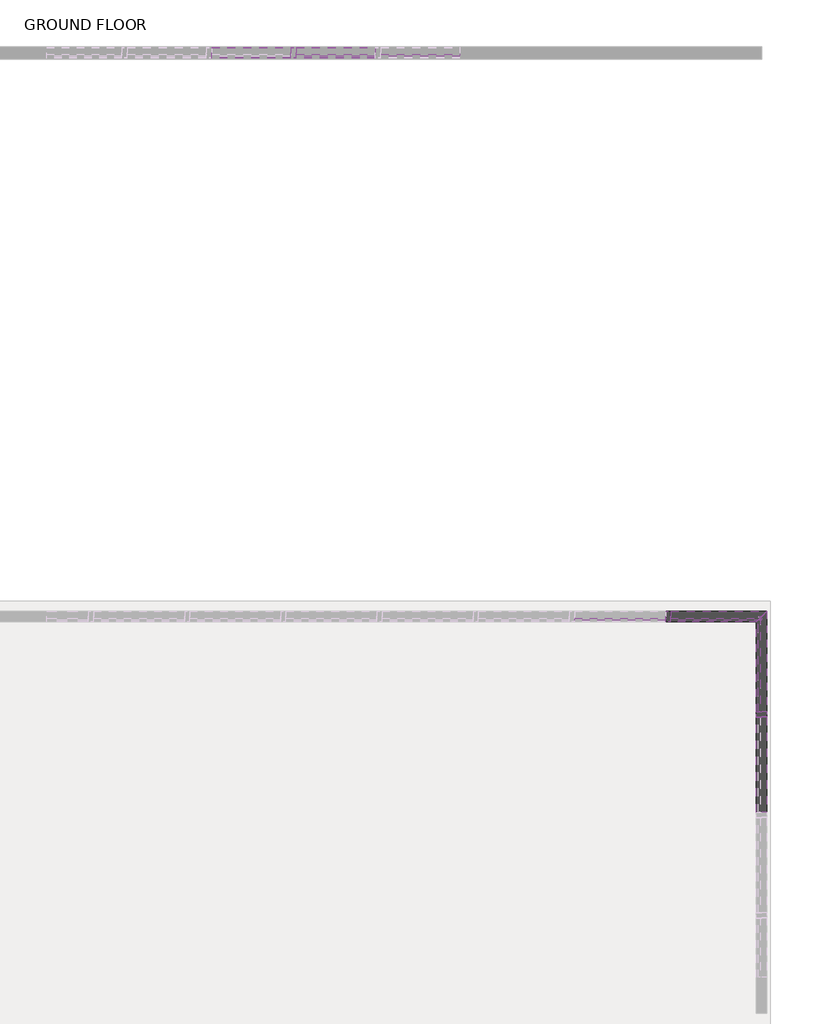
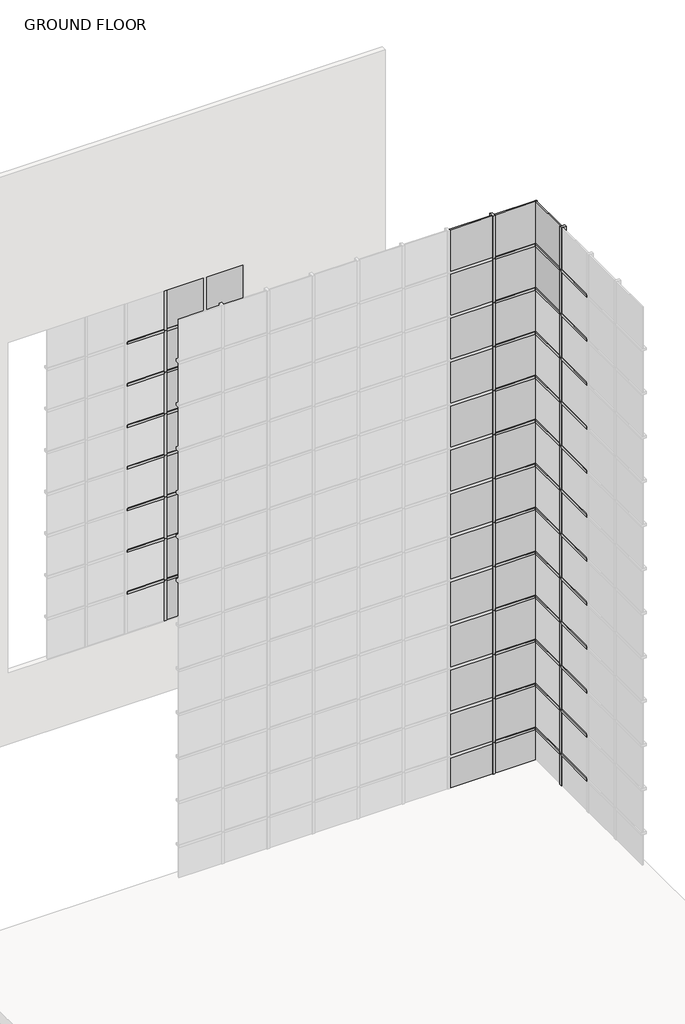
# One storey, part 14 of 16: 84 members, 44 plates.
"""IFC4 building model written with IfcOpenShell, lengths in millimetres."""

from ifc_helpers import new_model, si_unit, origin, place, context, project, spatial, transform, mapped, element, save
from components import member_b860638c, member_31fee25f, member_49b1bc66, member_1d29426d, member_637f24d3, member_76449a13, member_3df3cfcf, member_368818a6, system_panel_glazed_5cba32e5, system_panel_glazed_49652e9e, system_panel_glazed_6a711426

model = new_model("IFC4")

# Units and contexts
model_context = context("Model", 3, world=origin())
ifc_project = project(units=[si_unit("LENGTHUNIT", "METRE", prefix="MILLI")], contexts=[model_context])

# Site, building, storey
site = spatial("IfcSite", under=ifc_project)
building = spatial("IfcBuilding", under=site)
storey = spatial("IfcBuildingStorey", under=building, Name="GROUND FLOOR", Elevation=0.0)

# Members
placement = place(None, origin())
member_shape = member_b860638c(model_context)
element("IfcMember", 1, ObjectType="Rectangular Mullion : 2.5\" x 5\" rectangular", at=placement, inside=storey, context=model_context, shape_type="MappedRepresentation", body=[
    mapped(member_shape, transform((5962.6982466, 5184.6811965, 0.0), x_axis=(0.0, 1.0, 0.0), y_axis=(1.0, 0.0, 0.0), z_axis=(0.0, 0.0, -1.0))),
])
element("IfcMember", 2, ObjectType="Rectangular Mullion : 2.5\" x 5\" rectangular", at=placement, inside=storey, context=model_context, shape_type="MappedRepresentation", body=[
    mapped(member_shape, transform((4828.9790155, 6370.2261968, 0.0), x_axis=(-1.0, 0.0, 0.0), y_axis=(0.0, 1.0, 0.0), z_axis=(0.0, 0.0, -1.0))),
])
member_2_shape = member_31fee25f(model_context)
element("IfcMember", 3, ObjectType="Rectangular Mullion : 2.5\" x 5\" rectangular", at=placement, inside=storey, context=model_context, shape_type="MappedRepresentation", body=[
    mapped(member_2_shape, transform((5962.6982466, 5184.6811965, 1168.8884615), x_axis=(0.0, 1.0, 0.0), y_axis=(1.0, 0.0, 0.0), z_axis=(0.0, 0.0, -1.0))),
])
element("IfcMember", 4, ObjectType="Rectangular Mullion : 2.5\" x 5\" rectangular", at=placement, inside=storey, context=model_context, shape_type="MappedRepresentation", body=[
    mapped(member_2_shape, transform((5962.6982466, 5184.6811965, 2369.5269231), x_axis=(0.0, 1.0, 0.0), y_axis=(1.0, 0.0, 0.0), z_axis=(0.0, 0.0, -1.0))),
])
element("IfcMember", 5, ObjectType="Rectangular Mullion : 2.5\" x 5\" rectangular", at=placement, inside=storey, context=model_context, shape_type="MappedRepresentation", body=[
    mapped(member_2_shape, transform((5962.6982466, 5184.6811965, 3570.1653846), x_axis=(0.0, 1.0, 0.0), y_axis=(1.0, 0.0, 0.0), z_axis=(0.0, 0.0, -1.0))),
])
element("IfcMember", 6, ObjectType="Rectangular Mullion : 2.5\" x 5\" rectangular", at=placement, inside=storey, context=model_context, shape_type="MappedRepresentation", body=[
    mapped(member_2_shape, transform((5962.6982466, 5184.6811965, 4770.8038462), x_axis=(0.0, 1.0, 0.0), y_axis=(1.0, 0.0, 0.0), z_axis=(0.0, 0.0, -1.0))),
])
element("IfcMember", 7, ObjectType="Rectangular Mullion : 2.5\" x 5\" rectangular", at=placement, inside=storey, context=model_context, shape_type="MappedRepresentation", body=[
    mapped(member_2_shape, transform((5962.6982466, 5184.6811965, 5971.4423077), x_axis=(0.0, 1.0, 0.0), y_axis=(1.0, 0.0, 0.0), z_axis=(0.0, 0.0, -1.0))),
])
element("IfcMember", 8, ObjectType="Rectangular Mullion : 2.5\" x 5\" rectangular", at=placement, inside=storey, context=model_context, shape_type="MappedRepresentation", body=[
    mapped(member_2_shape, transform((5962.6982466, 5184.6811965, 7172.0807692), x_axis=(0.0, 1.0, 0.0), y_axis=(1.0, 0.0, 0.0), z_axis=(0.0, 0.0, -1.0))),
])
element("IfcMember", 9, ObjectType="Rectangular Mullion : 2.5\" x 5\" rectangular", at=placement, inside=storey, context=model_context, shape_type="MappedRepresentation", body=[
    mapped(member_2_shape, transform((5962.6982466, 5184.6811965, 8372.7192308), x_axis=(0.0, 1.0, 0.0), y_axis=(1.0, 0.0, 0.0), z_axis=(0.0, 0.0, -1.0))),
])
element("IfcMember", 10, ObjectType="Rectangular Mullion : 2.5\" x 5\" rectangular", at=placement, inside=storey, context=model_context, shape_type="MappedRepresentation", body=[
    mapped(member_2_shape, transform((5962.6982466, 5184.6811965, 9573.3576923), x_axis=(0.0, 1.0, 0.0), y_axis=(1.0, 0.0, 0.0), z_axis=(0.0, 0.0, -1.0))),
])
element("IfcMember", 11, ObjectType="Rectangular Mullion : 2.5\" x 5\" rectangular", at=placement, inside=storey, context=model_context, shape_type="MappedRepresentation", body=[
    mapped(member_2_shape, transform((5962.6982466, 5184.6811965, 10773.9961538), x_axis=(0.0, 1.0, 0.0), y_axis=(1.0, 0.0, 0.0), z_axis=(0.0, 0.0, -1.0))),
])
element("IfcMember", 12, ObjectType="Rectangular Mullion : 2.5\" x 5\" rectangular", at=placement, inside=storey, context=model_context, shape_type="MappedRepresentation", body=[
    mapped(member_2_shape, transform((5962.6982466, 5184.6811965, 11974.6346154), x_axis=(0.0, 1.0, 0.0), y_axis=(1.0, 0.0, 0.0), z_axis=(0.0, 0.0, -1.0))),
])
element("IfcMember", 13, ObjectType="Rectangular Mullion : 2.5\" x 5\" rectangular", at=placement, inside=storey, context=model_context, shape_type="MappedRepresentation", body=[
    mapped(member_2_shape, transform((5962.6982466, 5184.6811965, 13175.2730769), x_axis=(0.0, 1.0, 0.0), y_axis=(1.0, 0.0, 0.0), z_axis=(0.0, 0.0, -1.0))),
])
element("IfcMember", 14, ObjectType="Rectangular Mullion : 2.5\" x 5\" rectangular", at=placement, inside=storey, context=model_context, shape_type="MappedRepresentation", body=[
    mapped(member_2_shape, transform((4828.9790155, 6370.2261968, 1168.8884615), x_axis=(-1.0, 0.0, 0.0), y_axis=(0.0, 1.0, 0.0), z_axis=(0.0, 0.0, -1.0))),
])
element("IfcMember", 15, ObjectType="Rectangular Mullion : 2.5\" x 5\" rectangular", at=placement, inside=storey, context=model_context, shape_type="MappedRepresentation", body=[
    mapped(member_2_shape, transform((4828.9790155, 6370.2261968, 2369.5269231), x_axis=(-1.0, 0.0, 0.0), y_axis=(0.0, 1.0, 0.0), z_axis=(0.0, 0.0, -1.0))),
])
element("IfcMember", 16, ObjectType="Rectangular Mullion : 2.5\" x 5\" rectangular", at=placement, inside=storey, context=model_context, shape_type="MappedRepresentation", body=[
    mapped(member_2_shape, transform((4828.9790155, 6370.2261968, 3570.1653846), x_axis=(-1.0, 0.0, 0.0), y_axis=(0.0, 1.0, 0.0), z_axis=(0.0, 0.0, -1.0))),
])
element("IfcMember", 17, ObjectType="Rectangular Mullion : 2.5\" x 5\" rectangular", at=placement, inside=storey, context=model_context, shape_type="MappedRepresentation", body=[
    mapped(member_2_shape, transform((4828.9790155, 6370.2261968, 4770.8038462), x_axis=(-1.0, 0.0, 0.0), y_axis=(0.0, 1.0, 0.0), z_axis=(0.0, 0.0, -1.0))),
])
element("IfcMember", 18, ObjectType="Rectangular Mullion : 2.5\" x 5\" rectangular", at=placement, inside=storey, context=model_context, shape_type="MappedRepresentation", body=[
    mapped(member_2_shape, transform((4828.9790155, 6370.2261968, 5971.4423077), x_axis=(-1.0, 0.0, 0.0), y_axis=(0.0, 1.0, 0.0), z_axis=(0.0, 0.0, -1.0))),
])
element("IfcMember", 19, ObjectType="Rectangular Mullion : 2.5\" x 5\" rectangular", at=placement, inside=storey, context=model_context, shape_type="MappedRepresentation", body=[
    mapped(member_2_shape, transform((4828.9790155, 6370.2261968, 7172.0807692), x_axis=(-1.0, 0.0, 0.0), y_axis=(0.0, 1.0, 0.0), z_axis=(0.0, 0.0, -1.0))),
])
element("IfcMember", 20, ObjectType="Rectangular Mullion : 2.5\" x 5\" rectangular", at=placement, inside=storey, context=model_context, shape_type="MappedRepresentation", body=[
    mapped(member_2_shape, transform((4828.9790155, 6370.2261968, 8372.7192308), x_axis=(-1.0, 0.0, 0.0), y_axis=(0.0, 1.0, 0.0), z_axis=(0.0, 0.0, -1.0))),
])
element("IfcMember", 21, ObjectType="Rectangular Mullion : 2.5\" x 5\" rectangular", at=placement, inside=storey, context=model_context, shape_type="MappedRepresentation", body=[
    mapped(member_2_shape, transform((4828.9790155, 6370.2261968, 9573.3576923), x_axis=(-1.0, 0.0, 0.0), y_axis=(0.0, 1.0, 0.0), z_axis=(0.0, 0.0, -1.0))),
])
element("IfcMember", 22, ObjectType="Rectangular Mullion : 2.5\" x 5\" rectangular", at=placement, inside=storey, context=model_context, shape_type="MappedRepresentation", body=[
    mapped(member_2_shape, transform((4828.9790155, 6370.2261968, 10773.9961538), x_axis=(-1.0, 0.0, 0.0), y_axis=(0.0, 1.0, 0.0), z_axis=(0.0, 0.0, -1.0))),
])
element("IfcMember", 23, ObjectType="Rectangular Mullion : 2.5\" x 5\" rectangular", at=placement, inside=storey, context=model_context, shape_type="MappedRepresentation", body=[
    mapped(member_2_shape, transform((4828.9790155, 6370.2261968, 11974.6346154), x_axis=(-1.0, 0.0, 0.0), y_axis=(0.0, 1.0, 0.0), z_axis=(0.0, 0.0, -1.0))),
])
element("IfcMember", 24, ObjectType="Rectangular Mullion : 2.5\" x 5\" rectangular", at=placement, inside=storey, context=model_context, shape_type="MappedRepresentation", body=[
    mapped(member_2_shape, transform((4828.9790155, 6370.2261968, 13175.2730769), x_axis=(-1.0, 0.0, 0.0), y_axis=(0.0, 1.0, 0.0), z_axis=(0.0, 0.0, -1.0))),
])
element("IfcMember", 25, ObjectType="Rectangular Mullion : 2.5\" x 5\" rectangular", at=placement, inside=storey, context=model_context, shape_type="MappedRepresentation", body=[
    mapped(member_shape, transform((5962.6982466, 5184.6811965, 14375.9115385), x_axis=(0.0, 1.0, 0.0), y_axis=(1.0, 0.0, 0.0), z_axis=(0.0, 0.0, -1.0))),
])
element("IfcMember", 26, ObjectType="Rectangular Mullion : 2.5\" x 5\" rectangular", at=placement, inside=storey, context=model_context, shape_type="MappedRepresentation", body=[
    mapped(member_shape, transform((4828.9790155, 6370.2261968, 14375.9115385), x_axis=(-1.0, 0.0, 0.0), y_axis=(0.0, 1.0, 0.0), z_axis=(0.0, 0.0, -1.0))),
])
member_3_shape = member_49b1bc66(model_context)
element("IfcMember", 27, ObjectType="Rectangular Mullion : 2.5\" x 5\" rectangular", at=placement, inside=storey, context=model_context, shape_type="MappedRepresentation", body=[
    mapped(member_3_shape, transform((5962.6982466, 5152.9311965, 1168.8884615), x_axis=(0.0, 0.0, 1.0), y_axis=(1.0, 0.0, 0.0), z_axis=(0.0, 1.0, 0.0))),
])
element("IfcMember", 28, ObjectType="Rectangular Mullion : 2.5\" x 5\" rectangular", at=placement, inside=storey, context=model_context, shape_type="MappedRepresentation", body=[
    mapped(member_3_shape, transform((5962.6982466, 5152.9311965, 2369.5269231), x_axis=(0.0, 0.0, 1.0), y_axis=(1.0, 0.0, 0.0), z_axis=(0.0, 1.0, 0.0))),
])
element("IfcMember", 29, ObjectType="Rectangular Mullion : 2.5\" x 5\" rectangular", at=placement, inside=storey, context=model_context, shape_type="MappedRepresentation", body=[
    mapped(member_3_shape, transform((5962.6982466, 5152.9311965, 3570.1653846), x_axis=(0.0, 0.0, 1.0), y_axis=(1.0, 0.0, 0.0), z_axis=(0.0, 1.0, 0.0))),
])
element("IfcMember", 30, ObjectType="Rectangular Mullion : 2.5\" x 5\" rectangular", at=placement, inside=storey, context=model_context, shape_type="MappedRepresentation", body=[
    mapped(member_3_shape, transform((5962.6982466, 5152.9311965, 4770.8038462), x_axis=(0.0, 0.0, 1.0), y_axis=(1.0, 0.0, 0.0), z_axis=(0.0, 1.0, 0.0))),
])
element("IfcMember", 31, ObjectType="Rectangular Mullion : 2.5\" x 5\" rectangular", at=placement, inside=storey, context=model_context, shape_type="MappedRepresentation", body=[
    mapped(member_3_shape, transform((5962.6982466, 5152.9311965, 5971.4423077), x_axis=(0.0, 0.0, 1.0), y_axis=(1.0, 0.0, 0.0), z_axis=(0.0, 1.0, 0.0))),
])
element("IfcMember", 32, ObjectType="Rectangular Mullion : 2.5\" x 5\" rectangular", at=placement, inside=storey, context=model_context, shape_type="MappedRepresentation", body=[
    mapped(member_3_shape, transform((5962.6982466, 5152.9311965, 7172.0807692), x_axis=(0.0, 0.0, 1.0), y_axis=(1.0, 0.0, 0.0), z_axis=(0.0, 1.0, 0.0))),
])
element("IfcMember", 33, ObjectType="Rectangular Mullion : 2.5\" x 5\" rectangular", at=placement, inside=storey, context=model_context, shape_type="MappedRepresentation", body=[
    mapped(member_3_shape, transform((5962.6982466, 5152.9311965, 8372.7192308), x_axis=(0.0, 0.0, 1.0), y_axis=(1.0, 0.0, 0.0), z_axis=(0.0, 1.0, 0.0))),
])
element("IfcMember", 34, ObjectType="Rectangular Mullion : 2.5\" x 5\" rectangular", at=placement, inside=storey, context=model_context, shape_type="MappedRepresentation", body=[
    mapped(member_3_shape, transform((5962.6982466, 5152.9311965, 9573.3576923), x_axis=(0.0, 0.0, 1.0), y_axis=(1.0, 0.0, 0.0), z_axis=(0.0, 1.0, 0.0))),
])
element("IfcMember", 35, ObjectType="Rectangular Mullion : 2.5\" x 5\" rectangular", at=placement, inside=storey, context=model_context, shape_type="MappedRepresentation", body=[
    mapped(member_3_shape, transform((5962.6982466, 5152.9311965, 10773.9961538), x_axis=(0.0, 0.0, 1.0), y_axis=(1.0, 0.0, 0.0), z_axis=(0.0, 1.0, 0.0))),
])
element("IfcMember", 36, ObjectType="Rectangular Mullion : 2.5\" x 5\" rectangular", at=placement, inside=storey, context=model_context, shape_type="MappedRepresentation", body=[
    mapped(member_3_shape, transform((5962.6982466, 5152.9311965, 11974.6346154), x_axis=(0.0, 0.0, 1.0), y_axis=(1.0, 0.0, 0.0), z_axis=(0.0, 1.0, 0.0))),
])
element("IfcMember", 37, ObjectType="Rectangular Mullion : 2.5\" x 5\" rectangular", at=placement, inside=storey, context=model_context, shape_type="MappedRepresentation", body=[
    mapped(member_3_shape, transform((5962.6982466, 5152.9311965, 13175.2730769), x_axis=(0.0, 0.0, 1.0), y_axis=(1.0, 0.0, 0.0), z_axis=(0.0, 1.0, 0.0))),
])
element("IfcMember", 38, ObjectType="Rectangular Mullion : 2.5\" x 5\" rectangular", at=placement, inside=storey, context=model_context, shape_type="MappedRepresentation", body=[
    mapped(member_3_shape, transform((5962.6982466, 5152.9311965, 14375.9115385), x_axis=(0.0, 0.0, 1.0), y_axis=(1.0, 0.0, 0.0), z_axis=(0.0, 1.0, 0.0))),
])
member_4_shape = member_1d29426d(model_context)
element("IfcMember", 39, ObjectType="Rectangular Mullion : 2.5\" x 5\" rectangular", at=placement, inside=storey, context=model_context, shape_type="MappedRepresentation", body=[
    mapped(member_4_shape, transform((5962.6982466, 6370.2261968, 1168.8884615), x_axis=(0.0, 0.0, 1.0), y_axis=(1.0, 0.0, 0.0), z_axis=(0.0, 1.0, 0.0))),
])
element("IfcMember", 40, ObjectType="Rectangular Mullion : 2.5\" x 5\" rectangular", at=placement, inside=storey, context=model_context, shape_type="MappedRepresentation", body=[
    mapped(member_4_shape, transform((5962.6982466, 6370.2261968, 2369.5269231), x_axis=(0.0, 0.0, 1.0), y_axis=(1.0, 0.0, 0.0), z_axis=(0.0, 1.0, 0.0))),
])
element("IfcMember", 41, ObjectType="Rectangular Mullion : 2.5\" x 5\" rectangular", at=placement, inside=storey, context=model_context, shape_type="MappedRepresentation", body=[
    mapped(member_4_shape, transform((5962.6982466, 6370.2261968, 3570.1653846), x_axis=(0.0, 0.0, 1.0), y_axis=(1.0, 0.0, 0.0), z_axis=(0.0, 1.0, 0.0))),
])
element("IfcMember", 42, ObjectType="Rectangular Mullion : 2.5\" x 5\" rectangular", at=placement, inside=storey, context=model_context, shape_type="MappedRepresentation", body=[
    mapped(member_4_shape, transform((5962.6982466, 6370.2261968, 4770.8038462), x_axis=(0.0, 0.0, 1.0), y_axis=(1.0, 0.0, 0.0), z_axis=(0.0, 1.0, 0.0))),
])
element("IfcMember", 43, ObjectType="Rectangular Mullion : 2.5\" x 5\" rectangular", at=placement, inside=storey, context=model_context, shape_type="MappedRepresentation", body=[
    mapped(member_4_shape, transform((5962.6982466, 6370.2261968, 5971.4423077), x_axis=(0.0, 0.0, 1.0), y_axis=(1.0, 0.0, 0.0), z_axis=(0.0, 1.0, 0.0))),
])
element("IfcMember", 44, ObjectType="Rectangular Mullion : 2.5\" x 5\" rectangular", at=placement, inside=storey, context=model_context, shape_type="MappedRepresentation", body=[
    mapped(member_4_shape, transform((5962.6982466, 6370.2261968, 7172.0807692), x_axis=(0.0, 0.0, 1.0), y_axis=(1.0, 0.0, 0.0), z_axis=(0.0, 1.0, 0.0))),
])
element("IfcMember", 45, ObjectType="Rectangular Mullion : 2.5\" x 5\" rectangular", at=placement, inside=storey, context=model_context, shape_type="MappedRepresentation", body=[
    mapped(member_4_shape, transform((5962.6982466, 6370.2261968, 8372.7192308), x_axis=(0.0, 0.0, 1.0), y_axis=(1.0, 0.0, 0.0), z_axis=(0.0, 1.0, 0.0))),
])
element("IfcMember", 46, ObjectType="Rectangular Mullion : 2.5\" x 5\" rectangular", at=placement, inside=storey, context=model_context, shape_type="MappedRepresentation", body=[
    mapped(member_4_shape, transform((5962.6982466, 6370.2261968, 9573.3576923), x_axis=(0.0, 0.0, 1.0), y_axis=(1.0, 0.0, 0.0), z_axis=(0.0, 1.0, 0.0))),
])
element("IfcMember", 47, ObjectType="Rectangular Mullion : 2.5\" x 5\" rectangular", at=placement, inside=storey, context=model_context, shape_type="MappedRepresentation", body=[
    mapped(member_4_shape, transform((5962.6982466, 6370.2261968, 10773.9961538), x_axis=(0.0, 0.0, 1.0), y_axis=(1.0, 0.0, 0.0), z_axis=(0.0, 1.0, 0.0))),
])
element("IfcMember", 48, ObjectType="Rectangular Mullion : 2.5\" x 5\" rectangular", at=placement, inside=storey, context=model_context, shape_type="MappedRepresentation", body=[
    mapped(member_4_shape, transform((5962.6982466, 6370.2261968, 11974.6346154), x_axis=(0.0, 0.0, 1.0), y_axis=(1.0, 0.0, 0.0), z_axis=(0.0, 1.0, 0.0))),
])
element("IfcMember", 49, ObjectType="Rectangular Mullion : 2.5\" x 5\" rectangular", at=placement, inside=storey, context=model_context, shape_type="MappedRepresentation", body=[
    mapped(member_4_shape, transform((5962.6982466, 6370.2261968, 13175.2730769), x_axis=(0.0, 0.0, 1.0), y_axis=(1.0, 0.0, 0.0), z_axis=(0.0, 1.0, 0.0))),
])
element("IfcMember", 50, ObjectType="Rectangular Mullion : 2.5\" x 5\" rectangular", at=placement, inside=storey, context=model_context, shape_type="MappedRepresentation", body=[
    mapped(member_4_shape, transform((5962.6982466, 6370.2261968, 14375.9115385), x_axis=(0.0, 0.0, 1.0), y_axis=(1.0, 0.0, 0.0), z_axis=(0.0, 1.0, 0.0))),
])
member_5_shape = member_637f24d3(model_context)
element("IfcMember", 51, ObjectType="Rectangular Mullion : 2.5\" x 5\" rectangular", at=placement, inside=storey, context=model_context, shape_type="MappedRepresentation", body=[
    mapped(member_5_shape, transform((4860.7290155, 6370.2261968, 1168.8884615), x_axis=(0.0, 0.0, 1.0), y_axis=(0.0, 1.0, 0.0), z_axis=(-1.0, 0.0, 0.0))),
])
element("IfcMember", 52, ObjectType="Rectangular Mullion : 2.5\" x 5\" rectangular", at=placement, inside=storey, context=model_context, shape_type="MappedRepresentation", body=[
    mapped(member_5_shape, transform((4860.7290155, 6370.2261968, 2369.5269231), x_axis=(0.0, 0.0, 1.0), y_axis=(0.0, 1.0, 0.0), z_axis=(-1.0, 0.0, 0.0))),
])
element("IfcMember", 53, ObjectType="Rectangular Mullion : 2.5\" x 5\" rectangular", at=placement, inside=storey, context=model_context, shape_type="MappedRepresentation", body=[
    mapped(member_5_shape, transform((4860.7290155, 6370.2261968, 3570.1653846), x_axis=(0.0, 0.0, 1.0), y_axis=(0.0, 1.0, 0.0), z_axis=(-1.0, 0.0, 0.0))),
])
element("IfcMember", 54, ObjectType="Rectangular Mullion : 2.5\" x 5\" rectangular", at=placement, inside=storey, context=model_context, shape_type="MappedRepresentation", body=[
    mapped(member_5_shape, transform((4860.7290155, 6370.2261968, 4770.8038462), x_axis=(0.0, 0.0, 1.0), y_axis=(0.0, 1.0, 0.0), z_axis=(-1.0, 0.0, 0.0))),
])
element("IfcMember", 55, ObjectType="Rectangular Mullion : 2.5\" x 5\" rectangular", at=placement, inside=storey, context=model_context, shape_type="MappedRepresentation", body=[
    mapped(member_5_shape, transform((4860.7290155, 6370.2261968, 5971.4423077), x_axis=(0.0, 0.0, 1.0), y_axis=(0.0, 1.0, 0.0), z_axis=(-1.0, 0.0, 0.0))),
])
element("IfcMember", 56, ObjectType="Rectangular Mullion : 2.5\" x 5\" rectangular", at=placement, inside=storey, context=model_context, shape_type="MappedRepresentation", body=[
    mapped(member_5_shape, transform((4860.7290155, 6370.2261968, 7172.0807692), x_axis=(0.0, 0.0, 1.0), y_axis=(0.0, 1.0, 0.0), z_axis=(-1.0, 0.0, 0.0))),
])
element("IfcMember", 57, ObjectType="Rectangular Mullion : 2.5\" x 5\" rectangular", at=placement, inside=storey, context=model_context, shape_type="MappedRepresentation", body=[
    mapped(member_5_shape, transform((4860.7290155, 6370.2261968, 8372.7192308), x_axis=(0.0, 0.0, 1.0), y_axis=(0.0, 1.0, 0.0), z_axis=(-1.0, 0.0, 0.0))),
])
element("IfcMember", 58, ObjectType="Rectangular Mullion : 2.5\" x 5\" rectangular", at=placement, inside=storey, context=model_context, shape_type="MappedRepresentation", body=[
    mapped(member_5_shape, transform((4860.7290155, 6370.2261968, 9573.3576923), x_axis=(0.0, 0.0, 1.0), y_axis=(0.0, 1.0, 0.0), z_axis=(-1.0, 0.0, 0.0))),
])
element("IfcMember", 59, ObjectType="Rectangular Mullion : 2.5\" x 5\" rectangular", at=placement, inside=storey, context=model_context, shape_type="MappedRepresentation", body=[
    mapped(member_5_shape, transform((4860.7290155, 6370.2261968, 10773.9961538), x_axis=(0.0, 0.0, 1.0), y_axis=(0.0, 1.0, 0.0), z_axis=(-1.0, 0.0, 0.0))),
])
element("IfcMember", 60, ObjectType="Rectangular Mullion : 2.5\" x 5\" rectangular", at=placement, inside=storey, context=model_context, shape_type="MappedRepresentation", body=[
    mapped(member_5_shape, transform((4860.7290155, 6370.2261968, 11974.6346154), x_axis=(0.0, 0.0, 1.0), y_axis=(0.0, 1.0, 0.0), z_axis=(-1.0, 0.0, 0.0))),
])
element("IfcMember", 61, ObjectType="Rectangular Mullion : 2.5\" x 5\" rectangular", at=placement, inside=storey, context=model_context, shape_type="MappedRepresentation", body=[
    mapped(member_5_shape, transform((4860.7290155, 6370.2261968, 13175.2730769), x_axis=(0.0, 0.0, 1.0), y_axis=(0.0, 1.0, 0.0), z_axis=(-1.0, 0.0, 0.0))),
])
element("IfcMember", 62, ObjectType="Rectangular Mullion : 2.5\" x 5\" rectangular", at=placement, inside=storey, context=model_context, shape_type="MappedRepresentation", body=[
    mapped(member_5_shape, transform((4860.7290155, 6370.2261968, 14375.9115385), x_axis=(0.0, 0.0, 1.0), y_axis=(0.0, 1.0, 0.0), z_axis=(-1.0, 0.0, 0.0))),
])
member_6_shape = member_76449a13(model_context)
element("IfcMember", 63, ObjectType="Rectangular Mullion : 2.5\" x 5\" rectangular", at=placement, inside=storey, context=model_context, shape_type="MappedRepresentation", body=[
    mapped(member_6_shape, transform((258.6579457, 13200.7626438, 3045.6877023), x_axis=(0.0, 0.0, 1.0), y_axis=(0.0, -1.0, 0.0), z_axis=(1.0, 0.0, 0.0))),
])
element("IfcMember", 64, ObjectType="Rectangular Mullion : 2.5\" x 5\" rectangular", at=placement, inside=storey, context=model_context, shape_type="MappedRepresentation", body=[
    mapped(member_6_shape, transform((1282.5514531, 13200.7626438, 3045.6877023), x_axis=(0.0, 0.0, 1.0), y_axis=(0.0, -1.0, 0.0), z_axis=(1.0, 0.0, 0.0))),
])
element("IfcMember", 65, ObjectType="Rectangular Mullion : 2.5\" x 5\" rectangular", at=placement, inside=storey, context=model_context, shape_type="MappedRepresentation", body=[
    mapped(member_6_shape, transform((258.6579457, 13200.7626438, 4181.5290519), x_axis=(0.0, 0.0, 1.0), y_axis=(0.0, -1.0, 0.0), z_axis=(1.0, 0.0, 0.0))),
])
element("IfcMember", 66, ObjectType="Rectangular Mullion : 2.5\" x 5\" rectangular", at=placement, inside=storey, context=model_context, shape_type="MappedRepresentation", body=[
    mapped(member_6_shape, transform((1282.5514531, 13200.7626438, 4181.5290519), x_axis=(0.0, 0.0, 1.0), y_axis=(0.0, -1.0, 0.0), z_axis=(1.0, 0.0, 0.0))),
])
element("IfcMember", 67, ObjectType="Rectangular Mullion : 2.5\" x 5\" rectangular", at=placement, inside=storey, context=model_context, shape_type="MappedRepresentation", body=[
    mapped(member_6_shape, transform((258.6579457, 13200.7626438, 5317.3704015), x_axis=(0.0, 0.0, 1.0), y_axis=(0.0, -1.0, 0.0), z_axis=(1.0, 0.0, 0.0))),
])
element("IfcMember", 68, ObjectType="Rectangular Mullion : 2.5\" x 5\" rectangular", at=placement, inside=storey, context=model_context, shape_type="MappedRepresentation", body=[
    mapped(member_6_shape, transform((1282.5514531, 13200.7626438, 5317.3704015), x_axis=(0.0, 0.0, 1.0), y_axis=(0.0, -1.0, 0.0), z_axis=(1.0, 0.0, 0.0))),
])
element("IfcMember", 69, ObjectType="Rectangular Mullion : 2.5\" x 5\" rectangular", at=placement, inside=storey, context=model_context, shape_type="MappedRepresentation", body=[
    mapped(member_6_shape, transform((258.6579457, 13200.7626438, 6453.2117511), x_axis=(0.0, 0.0, 1.0), y_axis=(0.0, -1.0, 0.0), z_axis=(1.0, 0.0, 0.0))),
])
element("IfcMember", 70, ObjectType="Rectangular Mullion : 2.5\" x 5\" rectangular", at=placement, inside=storey, context=model_context, shape_type="MappedRepresentation", body=[
    mapped(member_6_shape, transform((1282.5514531, 13200.7626438, 6453.2117511), x_axis=(0.0, 0.0, 1.0), y_axis=(0.0, -1.0, 0.0), z_axis=(1.0, 0.0, 0.0))),
])
element("IfcMember", 71, ObjectType="Rectangular Mullion : 2.5\" x 5\" rectangular", at=placement, inside=storey, context=model_context, shape_type="MappedRepresentation", body=[
    mapped(member_6_shape, transform((258.6579457, 13200.7626438, 7589.0531007), x_axis=(0.0, 0.0, 1.0), y_axis=(0.0, -1.0, 0.0), z_axis=(1.0, 0.0, 0.0))),
])
element("IfcMember", 72, ObjectType="Rectangular Mullion : 2.5\" x 5\" rectangular", at=placement, inside=storey, context=model_context, shape_type="MappedRepresentation", body=[
    mapped(member_6_shape, transform((1282.5514531, 13200.7626438, 7589.0531007), x_axis=(0.0, 0.0, 1.0), y_axis=(0.0, -1.0, 0.0), z_axis=(1.0, 0.0, 0.0))),
])
element("IfcMember", 73, ObjectType="Rectangular Mullion : 2.5\" x 5\" rectangular", at=placement, inside=storey, context=model_context, shape_type="MappedRepresentation", body=[
    mapped(member_6_shape, transform((258.6579457, 13200.7626438, 8724.8944503), x_axis=(0.0, 0.0, 1.0), y_axis=(0.0, -1.0, 0.0), z_axis=(1.0, 0.0, 0.0))),
])
element("IfcMember", 74, ObjectType="Rectangular Mullion : 2.5\" x 5\" rectangular", at=placement, inside=storey, context=model_context, shape_type="MappedRepresentation", body=[
    mapped(member_6_shape, transform((1282.5514531, 13200.7626438, 8724.8944503), x_axis=(0.0, 0.0, 1.0), y_axis=(0.0, -1.0, 0.0), z_axis=(1.0, 0.0, 0.0))),
])
element("IfcMember", 75, ObjectType="Rectangular Mullion : 2.5\" x 5\" rectangular", at=placement, inside=storey, context=model_context, shape_type="MappedRepresentation", body=[
    mapped(member_6_shape, transform((258.6579457, 13200.7626438, 9860.7357999), x_axis=(0.0, 0.0, 1.0), y_axis=(0.0, -1.0, 0.0), z_axis=(1.0, 0.0, 0.0))),
])
element("IfcMember", 76, ObjectType="Rectangular Mullion : 2.5\" x 5\" rectangular", at=placement, inside=storey, context=model_context, shape_type="MappedRepresentation", body=[
    mapped(member_6_shape, transform((1282.5514531, 13200.7626438, 9860.7357999), x_axis=(0.0, 0.0, 1.0), y_axis=(0.0, -1.0, 0.0), z_axis=(1.0, 0.0, 0.0))),
])
member_7_shape = member_3df3cfcf(model_context)
element("IfcMember", 77, ObjectType="Rectangular Mullion : 2.5\" x 5\" rectangular", at=placement, inside=storey, context=model_context, shape_type="MappedRepresentation", body=[
    mapped(member_7_shape, transform((290.4079457, 13200.7626438, 1941.5963527), x_axis=(1.0, 0.0, 0.0), y_axis=(0.0, -1.0, 0.0), z_axis=(0.0, 0.0, -1.0))),
])
member_8_shape = member_368818a6(model_context)
element("IfcMember", 78, ObjectType="Rectangular Mullion : 2.5\" x 5\" rectangular", at=placement, inside=storey, context=model_context, shape_type="MappedRepresentation", body=[
    mapped(member_8_shape, transform((290.4079457, 13200.7626438, 3045.6877023), x_axis=(1.0, 0.0, 0.0), y_axis=(0.0, -1.0, 0.0), z_axis=(0.0, 0.0, -1.0))),
])
element("IfcMember", 79, ObjectType="Rectangular Mullion : 2.5\" x 5\" rectangular", at=placement, inside=storey, context=model_context, shape_type="MappedRepresentation", body=[
    mapped(member_8_shape, transform((290.4079457, 13200.7626438, 4181.5290519), x_axis=(1.0, 0.0, 0.0), y_axis=(0.0, -1.0, 0.0), z_axis=(0.0, 0.0, -1.0))),
])
element("IfcMember", 80, ObjectType="Rectangular Mullion : 2.5\" x 5\" rectangular", at=placement, inside=storey, context=model_context, shape_type="MappedRepresentation", body=[
    mapped(member_8_shape, transform((290.4079457, 13200.7626438, 5317.3704015), x_axis=(1.0, 0.0, 0.0), y_axis=(0.0, -1.0, 0.0), z_axis=(0.0, 0.0, -1.0))),
])
element("IfcMember", 81, ObjectType="Rectangular Mullion : 2.5\" x 5\" rectangular", at=placement, inside=storey, context=model_context, shape_type="MappedRepresentation", body=[
    mapped(member_8_shape, transform((290.4079457, 13200.7626438, 6453.2117511), x_axis=(1.0, 0.0, 0.0), y_axis=(0.0, -1.0, 0.0), z_axis=(0.0, 0.0, -1.0))),
])
element("IfcMember", 82, ObjectType="Rectangular Mullion : 2.5\" x 5\" rectangular", at=placement, inside=storey, context=model_context, shape_type="MappedRepresentation", body=[
    mapped(member_8_shape, transform((290.4079457, 13200.7626438, 7589.0531007), x_axis=(1.0, 0.0, 0.0), y_axis=(0.0, -1.0, 0.0), z_axis=(0.0, 0.0, -1.0))),
])
element("IfcMember", 83, ObjectType="Rectangular Mullion : 2.5\" x 5\" rectangular", at=placement, inside=storey, context=model_context, shape_type="MappedRepresentation", body=[
    mapped(member_8_shape, transform((290.4079457, 13200.7626438, 8724.8944503), x_axis=(1.0, 0.0, 0.0), y_axis=(0.0, -1.0, 0.0), z_axis=(0.0, 0.0, -1.0))),
])
element("IfcMember", 84, ObjectType="Rectangular Mullion : 2.5\" x 5\" rectangular", at=placement, inside=storey, context=model_context, shape_type="MappedRepresentation", body=[
    mapped(member_7_shape, transform((290.4079457, 13200.7626438, 9860.7357999), x_axis=(1.0, 0.0, 0.0), y_axis=(0.0, -1.0, 0.0), z_axis=(0.0, 0.0, -1.0))),
])

# Plates
system_panel_glazed_shape = system_panel_glazed_5cba32e5(model_context)
element("IfcPlate", 85, ObjectType="System Panel : Glazed", at=placement, inside=storey, context=model_context, shape_type="MappedRepresentation", body=[
    mapped(system_panel_glazed_shape, transform((5411.7136311, 6370.2261968, 0.0), x_axis=(-1.0, 0.0, 0.0), y_axis=(0.0, -1.0, 0.0), z_axis=(0.0, 0.0, 1.0))),
])
element("IfcPlate", 86, ObjectType="System Panel : Glazed", at=placement, inside=storey, context=model_context, shape_type="MappedRepresentation", body=[
    mapped(system_panel_glazed_shape, transform((4246.2444002, 6370.2261968, 0.0), x_axis=(-1.0, 0.0, 0.0), y_axis=(0.0, -1.0, 0.0), z_axis=(0.0, 0.0, 1.0))),
])
element("IfcPlate", 87, ObjectType="System Panel : Glazed", at=placement, inside=storey, context=model_context, shape_type="MappedRepresentation", body=[
    mapped(system_panel_glazed_shape, transform((5411.7136311, 6370.2261968, 1200.6384615), x_axis=(-1.0, 0.0, 0.0), y_axis=(0.0, -1.0, 0.0), z_axis=(0.0, 0.0, 1.0))),
])
element("IfcPlate", 88, ObjectType="System Panel : Glazed", at=placement, inside=storey, context=model_context, shape_type="MappedRepresentation", body=[
    mapped(system_panel_glazed_shape, transform((4246.2444002, 6370.2261968, 1200.6384615), x_axis=(-1.0, 0.0, 0.0), y_axis=(0.0, -1.0, 0.0), z_axis=(0.0, 0.0, 1.0))),
])
element("IfcPlate", 89, ObjectType="System Panel : Glazed", at=placement, inside=storey, context=model_context, shape_type="MappedRepresentation", body=[
    mapped(system_panel_glazed_shape, transform((5411.7136311, 6370.2261968, 2401.2769231), x_axis=(-1.0, 0.0, 0.0), y_axis=(0.0, -1.0, 0.0), z_axis=(0.0, 0.0, 1.0))),
])
element("IfcPlate", 90, ObjectType="System Panel : Glazed", at=placement, inside=storey, context=model_context, shape_type="MappedRepresentation", body=[
    mapped(system_panel_glazed_shape, transform((4246.2444002, 6370.2261968, 2401.2769231), x_axis=(-1.0, 0.0, 0.0), y_axis=(0.0, -1.0, 0.0), z_axis=(0.0, 0.0, 1.0))),
])
element("IfcPlate", 91, ObjectType="System Panel : Glazed", at=placement, inside=storey, context=model_context, shape_type="MappedRepresentation", body=[
    mapped(system_panel_glazed_shape, transform((5411.7136311, 6370.2261968, 3601.9153846), x_axis=(-1.0, 0.0, 0.0), y_axis=(0.0, -1.0, 0.0), z_axis=(0.0, 0.0, 1.0))),
])
element("IfcPlate", 92, ObjectType="System Panel : Glazed", at=placement, inside=storey, context=model_context, shape_type="MappedRepresentation", body=[
    mapped(system_panel_glazed_shape, transform((4246.2444002, 6370.2261968, 3601.9153846), x_axis=(-1.0, 0.0, 0.0), y_axis=(0.0, -1.0, 0.0), z_axis=(0.0, 0.0, 1.0))),
])
element("IfcPlate", 93, ObjectType="System Panel : Glazed", at=placement, inside=storey, context=model_context, shape_type="MappedRepresentation", body=[
    mapped(system_panel_glazed_shape, transform((5411.7136311, 6370.2261968, 4802.5538462), x_axis=(-1.0, 0.0, 0.0), y_axis=(0.0, -1.0, 0.0), z_axis=(0.0, 0.0, 1.0))),
])
element("IfcPlate", 94, ObjectType="System Panel : Glazed", at=placement, inside=storey, context=model_context, shape_type="MappedRepresentation", body=[
    mapped(system_panel_glazed_shape, transform((4246.2444002, 6370.2261968, 4802.5538462), x_axis=(-1.0, 0.0, 0.0), y_axis=(0.0, -1.0, 0.0), z_axis=(0.0, 0.0, 1.0))),
])
element("IfcPlate", 95, ObjectType="System Panel : Glazed", at=placement, inside=storey, context=model_context, shape_type="MappedRepresentation", body=[
    mapped(system_panel_glazed_shape, transform((5411.7136311, 6370.2261968, 6003.1923077), x_axis=(-1.0, 0.0, 0.0), y_axis=(0.0, -1.0, 0.0), z_axis=(0.0, 0.0, 1.0))),
])
element("IfcPlate", 96, ObjectType="System Panel : Glazed", at=placement, inside=storey, context=model_context, shape_type="MappedRepresentation", body=[
    mapped(system_panel_glazed_shape, transform((4246.2444002, 6370.2261968, 6003.1923077), x_axis=(-1.0, 0.0, 0.0), y_axis=(0.0, -1.0, 0.0), z_axis=(0.0, 0.0, 1.0))),
])
element("IfcPlate", 97, ObjectType="System Panel : Glazed", at=placement, inside=storey, context=model_context, shape_type="MappedRepresentation", body=[
    mapped(system_panel_glazed_shape, transform((5411.7136311, 6370.2261968, 7203.8307692), x_axis=(-1.0, 0.0, 0.0), y_axis=(0.0, -1.0, 0.0), z_axis=(0.0, 0.0, 1.0))),
])
element("IfcPlate", 98, ObjectType="System Panel : Glazed", at=placement, inside=storey, context=model_context, shape_type="MappedRepresentation", body=[
    mapped(system_panel_glazed_shape, transform((4246.2444002, 6370.2261968, 7203.8307692), x_axis=(-1.0, 0.0, 0.0), y_axis=(0.0, -1.0, 0.0), z_axis=(0.0, 0.0, 1.0))),
])
element("IfcPlate", 99, ObjectType="System Panel : Glazed", at=placement, inside=storey, context=model_context, shape_type="MappedRepresentation", body=[
    mapped(system_panel_glazed_shape, transform((5411.7136311, 6370.2261968, 8404.4692308), x_axis=(-1.0, 0.0, 0.0), y_axis=(0.0, -1.0, 0.0), z_axis=(0.0, 0.0, 1.0))),
])
element("IfcPlate", 100, ObjectType="System Panel : Glazed", at=placement, inside=storey, context=model_context, shape_type="MappedRepresentation", body=[
    mapped(system_panel_glazed_shape, transform((4246.2444002, 6370.2261968, 8404.4692308), x_axis=(-1.0, 0.0, 0.0), y_axis=(0.0, -1.0, 0.0), z_axis=(0.0, 0.0, 1.0))),
])
element("IfcPlate", 101, ObjectType="System Panel : Glazed", at=placement, inside=storey, context=model_context, shape_type="MappedRepresentation", body=[
    mapped(system_panel_glazed_shape, transform((5411.7136311, 6370.2261968, 9605.1076923), x_axis=(-1.0, 0.0, 0.0), y_axis=(0.0, -1.0, 0.0), z_axis=(0.0, 0.0, 1.0))),
])
element("IfcPlate", 102, ObjectType="System Panel : Glazed", at=placement, inside=storey, context=model_context, shape_type="MappedRepresentation", body=[
    mapped(system_panel_glazed_shape, transform((4246.2444002, 6370.2261968, 9605.1076923), x_axis=(-1.0, 0.0, 0.0), y_axis=(0.0, -1.0, 0.0), z_axis=(0.0, 0.0, 1.0))),
])
element("IfcPlate", 103, ObjectType="System Panel : Glazed", at=placement, inside=storey, context=model_context, shape_type="MappedRepresentation", body=[
    mapped(system_panel_glazed_shape, transform((5411.7136311, 6370.2261968, 10805.7461538), x_axis=(-1.0, 0.0, 0.0), y_axis=(0.0, -1.0, 0.0), z_axis=(0.0, 0.0, 1.0))),
])
element("IfcPlate", 104, ObjectType="System Panel : Glazed", at=placement, inside=storey, context=model_context, shape_type="MappedRepresentation", body=[
    mapped(system_panel_glazed_shape, transform((4246.2444002, 6370.2261968, 10805.7461538), x_axis=(-1.0, 0.0, 0.0), y_axis=(0.0, -1.0, 0.0), z_axis=(0.0, 0.0, 1.0))),
])
element("IfcPlate", 105, ObjectType="System Panel : Glazed", at=placement, inside=storey, context=model_context, shape_type="MappedRepresentation", body=[
    mapped(system_panel_glazed_shape, transform((5411.7136311, 6370.2261968, 12006.3846154), x_axis=(-1.0, 0.0, 0.0), y_axis=(0.0, -1.0, 0.0), z_axis=(0.0, 0.0, 1.0))),
])
element("IfcPlate", 106, ObjectType="System Panel : Glazed", at=placement, inside=storey, context=model_context, shape_type="MappedRepresentation", body=[
    mapped(system_panel_glazed_shape, transform((4246.2444002, 6370.2261968, 12006.3846154), x_axis=(-1.0, 0.0, 0.0), y_axis=(0.0, -1.0, 0.0), z_axis=(0.0, 0.0, 1.0))),
])
element("IfcPlate", 107, ObjectType="System Panel : Glazed", at=placement, inside=storey, context=model_context, shape_type="MappedRepresentation", body=[
    mapped(system_panel_glazed_shape, transform((5411.7136311, 6370.2261968, 13207.0230769), x_axis=(-1.0, 0.0, 0.0), y_axis=(0.0, -1.0, 0.0), z_axis=(0.0, 0.0, 1.0))),
])
element("IfcPlate", 108, ObjectType="System Panel : Glazed", at=placement, inside=storey, context=model_context, shape_type="MappedRepresentation", body=[
    mapped(system_panel_glazed_shape, transform((4246.2444002, 6370.2261968, 13207.0230769), x_axis=(-1.0, 0.0, 0.0), y_axis=(0.0, -1.0, 0.0), z_axis=(0.0, 0.0, 1.0))),
])
element("IfcPlate", 109, ObjectType="System Panel : Glazed", at=placement, inside=storey, context=model_context, shape_type="MappedRepresentation", body=[
    mapped(system_panel_glazed_shape, transform((5411.7136311, 6370.2261968, 14407.6615385), x_axis=(-1.0, 0.0, 0.0), y_axis=(0.0, -1.0, 0.0), z_axis=(0.0, 0.0, 1.0))),
])
element("IfcPlate", 110, ObjectType="System Panel : Glazed", at=placement, inside=storey, context=model_context, shape_type="MappedRepresentation", body=[
    mapped(system_panel_glazed_shape, transform((4246.2444002, 6370.2261968, 14407.6615385), x_axis=(-1.0, 0.0, 0.0), y_axis=(0.0, -1.0, 0.0), z_axis=(0.0, 0.0, 1.0))),
])
system_panel_glazed_2_shape = system_panel_glazed_49652e9e(model_context)
element("IfcPlate", 111, ObjectType="System Panel : Glazed", at=placement, inside=storey, context=model_context, shape_type="MappedRepresentation", body=[
    mapped(system_panel_glazed_2_shape, transform((5962.6982466, 5793.3286967, 13207.0230769), x_axis=(0.0, 1.0, 0.0), y_axis=(-1.0, 0.0, 0.0), z_axis=(0.0, 0.0, 1.0))),
])
element("IfcPlate", 112, ObjectType="System Panel : Glazed", at=placement, inside=storey, context=model_context, shape_type="MappedRepresentation", body=[
    mapped(system_panel_glazed_2_shape, transform((5962.6982466, 5793.3286967, 14407.6615385), x_axis=(0.0, 1.0, 0.0), y_axis=(-1.0, 0.0, 0.0), z_axis=(0.0, 0.0, 1.0))),
])
system_panel_glazed_3_shape = system_panel_glazed_6a711426(model_context)
element("IfcPlate", 113, ObjectType="System Panel : Glazed", at=placement, inside=storey, context=model_context, shape_type="MappedRepresentation", body=[
    mapped(system_panel_glazed_3_shape, transform((802.3546994, 13200.7626438, 1941.5963527), x_axis=(1.0, 0.0, 0.0), y_axis=(0.0, 1.0, 0.0), z_axis=(0.0, 0.0, 1.0))),
])
element("IfcPlate", 114, ObjectType="System Panel : Glazed", at=placement, inside=storey, context=model_context, shape_type="MappedRepresentation", body=[
    mapped(system_panel_glazed_3_shape, transform((1826.2482069, 13200.7626438, 1941.5963527), x_axis=(1.0, 0.0, 0.0), y_axis=(0.0, 1.0, 0.0), z_axis=(0.0, 0.0, 1.0))),
])
element("IfcPlate", 115, ObjectType="System Panel : Glazed", at=placement, inside=storey, context=model_context, shape_type="MappedRepresentation", body=[
    mapped(system_panel_glazed_3_shape, transform((802.3546994, 13200.7626438, 3077.4377023), x_axis=(1.0, 0.0, 0.0), y_axis=(0.0, 1.0, 0.0), z_axis=(0.0, 0.0, 1.0))),
])
element("IfcPlate", 116, ObjectType="System Panel : Glazed", at=placement, inside=storey, context=model_context, shape_type="MappedRepresentation", body=[
    mapped(system_panel_glazed_3_shape, transform((1826.2482069, 13200.7626438, 3077.4377023), x_axis=(1.0, 0.0, 0.0), y_axis=(0.0, 1.0, 0.0), z_axis=(0.0, 0.0, 1.0))),
])
element("IfcPlate", 117, ObjectType="System Panel : Glazed", at=placement, inside=storey, context=model_context, shape_type="MappedRepresentation", body=[
    mapped(system_panel_glazed_3_shape, transform((802.3546994, 13200.7626438, 4213.2790519), x_axis=(1.0, 0.0, 0.0), y_axis=(0.0, 1.0, 0.0), z_axis=(0.0, 0.0, 1.0))),
])
element("IfcPlate", 118, ObjectType="System Panel : Glazed", at=placement, inside=storey, context=model_context, shape_type="MappedRepresentation", body=[
    mapped(system_panel_glazed_3_shape, transform((1826.2482069, 13200.7626438, 4213.2790519), x_axis=(1.0, 0.0, 0.0), y_axis=(0.0, 1.0, 0.0), z_axis=(0.0, 0.0, 1.0))),
])
element("IfcPlate", 119, ObjectType="System Panel : Glazed", at=placement, inside=storey, context=model_context, shape_type="MappedRepresentation", body=[
    mapped(system_panel_glazed_3_shape, transform((802.3546994, 13200.7626438, 5349.1204015), x_axis=(1.0, 0.0, 0.0), y_axis=(0.0, 1.0, 0.0), z_axis=(0.0, 0.0, 1.0))),
])
element("IfcPlate", 120, ObjectType="System Panel : Glazed", at=placement, inside=storey, context=model_context, shape_type="MappedRepresentation", body=[
    mapped(system_panel_glazed_3_shape, transform((1826.2482069, 13200.7626438, 5349.1204015), x_axis=(1.0, 0.0, 0.0), y_axis=(0.0, 1.0, 0.0), z_axis=(0.0, 0.0, 1.0))),
])
element("IfcPlate", 121, ObjectType="System Panel : Glazed", at=placement, inside=storey, context=model_context, shape_type="MappedRepresentation", body=[
    mapped(system_panel_glazed_3_shape, transform((802.3546994, 13200.7626438, 6484.9617511), x_axis=(1.0, 0.0, 0.0), y_axis=(0.0, 1.0, 0.0), z_axis=(0.0, 0.0, 1.0))),
])
element("IfcPlate", 122, ObjectType="System Panel : Glazed", at=placement, inside=storey, context=model_context, shape_type="MappedRepresentation", body=[
    mapped(system_panel_glazed_3_shape, transform((1826.2482069, 13200.7626438, 6484.9617511), x_axis=(1.0, 0.0, 0.0), y_axis=(0.0, 1.0, 0.0), z_axis=(0.0, 0.0, 1.0))),
])
element("IfcPlate", 123, ObjectType="System Panel : Glazed", at=placement, inside=storey, context=model_context, shape_type="MappedRepresentation", body=[
    mapped(system_panel_glazed_3_shape, transform((802.3546994, 13200.7626438, 7620.8031007), x_axis=(1.0, 0.0, 0.0), y_axis=(0.0, 1.0, 0.0), z_axis=(0.0, 0.0, 1.0))),
])
element("IfcPlate", 124, ObjectType="System Panel : Glazed", at=placement, inside=storey, context=model_context, shape_type="MappedRepresentation", body=[
    mapped(system_panel_glazed_3_shape, transform((1826.2482069, 13200.7626438, 7620.8031007), x_axis=(1.0, 0.0, 0.0), y_axis=(0.0, 1.0, 0.0), z_axis=(0.0, 0.0, 1.0))),
])
element("IfcPlate", 125, ObjectType="System Panel : Glazed", at=placement, inside=storey, context=model_context, shape_type="MappedRepresentation", body=[
    mapped(system_panel_glazed_3_shape, transform((802.3546994, 13200.7626438, 8756.6444503), x_axis=(1.0, 0.0, 0.0), y_axis=(0.0, 1.0, 0.0), z_axis=(0.0, 0.0, 1.0))),
])
element("IfcPlate", 126, ObjectType="System Panel : Glazed", at=placement, inside=storey, context=model_context, shape_type="MappedRepresentation", body=[
    mapped(system_panel_glazed_3_shape, transform((1826.2482069, 13200.7626438, 8756.6444503), x_axis=(1.0, 0.0, 0.0), y_axis=(0.0, 1.0, 0.0), z_axis=(0.0, 0.0, 1.0))),
])
element("IfcPlate", 127, ObjectType="System Panel : Glazed", at=placement, inside=storey, context=model_context, shape_type="MappedRepresentation", body=[
    mapped(system_panel_glazed_3_shape, transform((802.3546994, 13200.7626438, 9892.4857999), x_axis=(1.0, 0.0, 0.0), y_axis=(0.0, 1.0, 0.0), z_axis=(0.0, 0.0, 1.0))),
])
element("IfcPlate", 128, ObjectType="System Panel : Glazed", at=placement, inside=storey, context=model_context, shape_type="MappedRepresentation", body=[
    mapped(system_panel_glazed_3_shape, transform((1826.2482069, 13200.7626438, 9892.4857999), x_axis=(1.0, 0.0, 0.0), y_axis=(0.0, 1.0, 0.0), z_axis=(0.0, 0.0, 1.0))),
])

save(model, "model.ifc")

# Revit data of these elements
# Type "Rectangular Mullion : 2.5\" x 5\" rectangular"
#   built-in parameter 1007304 = 0.416667 (stored number, unit not read)
#   built-in parameter 1007301 = 0.104167 (stored number, unit not read)
#   built-in parameter 1007300 = 0.104167 (stored number, unit not read)
# Type "System Panel : Glazed"
#   Construction Type Id = "GSP4R"
#   Analytic Construction = "1/8 in Pilkington single glazing"
#   Visual Light Transmittance = 0.9
#   Solar Heat Gain Coefficient = 0.86
#   Heat Transfer Coefficient (U) = 1.18115 BTU/(h·ft²·°F)
#   Define Thermal Properties by = 1
# Elements 1, 2, 3, 4, 5, 6, 7, 8, 9, 10, 11, 12, 13, 14, 15, 16, 17, 18, 19, 20, 21, 22, 23, 24, 25, 26, 27, 28, 29, 30, 31, 32, 33, 34, 35, 36, 37, 38, 39, 40, 41, 42, 43, 44, 45, 46, 47, 48, 49, 50, 51, 52, 53, 54, 55, 56, 57, 58, 59, 60, 61, 62, 63, 64, 65, 66, 67, 68, 69, 70, 71, 72, 73, 74, 75, 76, 77, 78, 79, 80, 81, 82, 83, 84 (IfcMember, "Rectangular Mullion : 2.5\" x 5\" rectangular")
#   Phase Created = New Construction
#   Materials on its faces: "Aluminum"
# Elements 85, 86, 87, 88, 89, 90, 91, 92, 93, 94, 95, 96, 97, 98, 99, 100, 101, 102, 103, 104, 105, 106, 107, 108, 109, 110, 111, 112, 113, 114, 115, 116, 117, 118, 119, 120, 121, 122, 123, 124, 125, 126, 127, 128 (IfcPlate, "System Panel : Glazed")
#   Phase Created = New Construction
#   Materials on its faces: "Glass"
# Materials
#   "Aluminum": class "Metal", colour RGB 247 247 247, transparency 0, Description = "Aluminum 6061", Cost = 0
#   "Glass": class "Glass", colour RGB 0 128 192, transparency 0.75, Description = "Soda Lime Glass", Cost = 0
